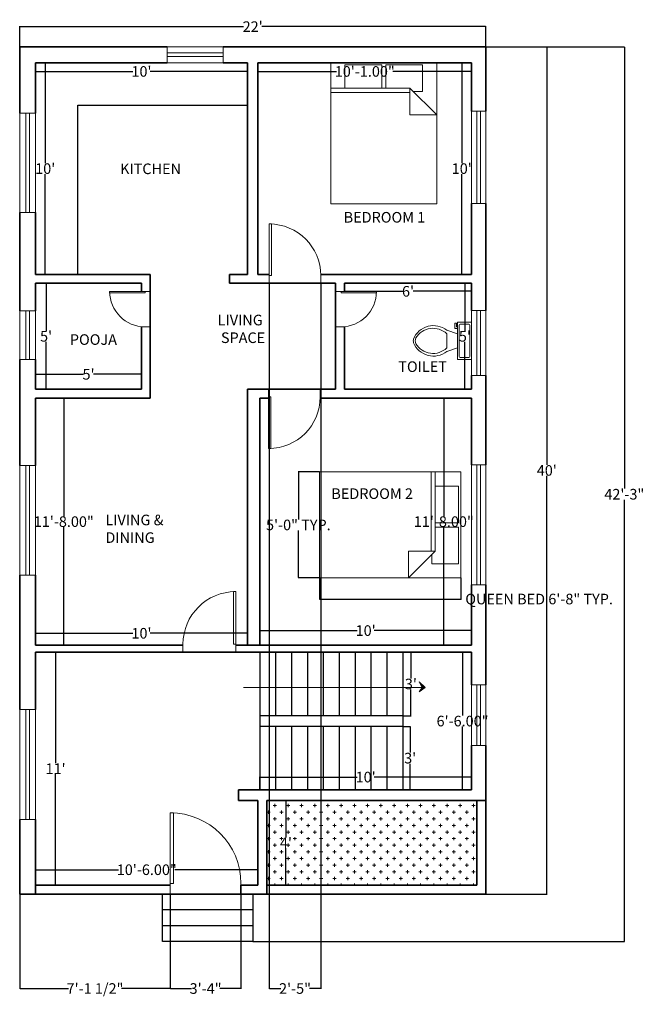
# Model space of a CAD drawing. Units: inches. Extents: x 14 to 1508, y -30 to 806.
# Tile 4 of 4: x 1154 to 1508, y -30 to 528. Entities that reach past the tile are written whole.
import ezdxf

# ---------------------------------------------------------------- set-up
doc = ezdxf.new("R2010")
doc.units = ezdxf.units.IN
doc.header["$MEASUREMENT"] = 0
for name, color, linetype, lineweight in [('A-ANNO-DIMS', 6, 'Continuous', 18), ('A-ANNO-SYMB', 2, 'Continuous', 18), ('A-AREA-IDEN', 3, 'Continuous', 18), ('A-DOOR', 4, 'Continuous', 18), ('A-FLOR-CASE', 8, 'Continuous', 25), ('A-FLOR-FIXT', 8, 'Continuous', 18), ('A-FLOR-PATT', 3, 'Continuous', 13), ('A-FLOR-STRS', 7, 'Continuous', 25), ('A-FURN', 8, 'Continuous', 18), ('A-GLAZ', 4, 'Continuous', 18), ('A-WALL', 7, 'Continuous', 35)]:
    doc.layers.add(name, color=color, linetype=linetype, lineweight=lineweight)
doc.styles.get("Standard").update_dxf_attribs({"font": 'arial.ttf'})
doc.dimstyles.get("Standard").update_dxf_attribs({"dimtxt": 6, "dimasz": 0.18, "dimexe": 0.18, "dimexo": 0.0625, "dimgap": 0.09, "dimtad": 0, "dimtih": 1, "dimtoh": 1, "dimzin": 0, "dimdsep": 46, "dimlunit": 3, "dimtxsty": 'Standard', "dimcen": 0.09, "dimadec": 0, "dimazin": 0, "dimtfac": 1, "dimtofl": 0, "dimtmove": 0, "dimatfit": 3, "dimfxl": 1, "dimtolj": 1, "dimtzin": 0, "dimarcsym": 0})

# ---------------------------------------------------------------- blocks, each defined once
blk = doc.blocks.new('*D55')
at = {"layer": 'A-ANNO-DIMS', "color": 0, "lineweight": -2, "transparency": 16777216}
for p, q in [((1370.88, 169.37), (1375.62, 169.37)), ((1375.44, 169.19), (1375.44, 154.52)), ((1375.44, 133.55), (1375.44, 148.21)), ((1370.88, 133.37), (1375.62, 133.37))]:
    blk.add_line(p, q, dxfattribs=at)
at = {"layer": 'A-ANNO-DIMS', "color": 0, "transparency": 16777216}
for points in [[(1375.41, 169.19), (1375.47, 169.19), (1375.44, 169.37)], [(1375.41, 133.55), (1375.47, 133.55), (1375.44, 133.37)]]:
    blk.add_solid(points, dxfattribs=at)
at = {"layer": 'Defpoints', "color": 0, "transparency": 16777216}
for p in [(1370.82, 169.37), (1375.44, 169.37), (1370.82, 133.37)]:
    blk.add_point(p, dxfattribs=at)
at = {"layer": 'A-ANNO-DIMS', "color": 0, "transparency": 16777216, "insert": (1375.44, 151.37), "char_height": 6, "attachment_point": 5}
blk.add_mtext("\\A1;3'", dxfattribs=at)
blk = doc.blocks.new('*D56')
at = {"layer": 'A-ANNO-DIMS', "color": 0, "lineweight": -2, "transparency": 16777216}
for p, q in [((1370.88, 127.37), (1375.22, 127.37)), ((1375.04, 127.19), (1375.04, 112.52)), ((1375.04, 91.55), (1375.04, 106.21)), ((1370.88, 91.37), (1375.22, 91.37))]:
    blk.add_line(p, q, dxfattribs=at)
at = {"layer": 'A-ANNO-DIMS', "color": 0, "transparency": 16777216}
for points in [[(1375.01, 127.19), (1375.07, 127.19), (1375.04, 127.37)], [(1375.01, 91.55), (1375.07, 91.55), (1375.04, 91.37)]]:
    blk.add_solid(points, dxfattribs=at)
at = {"layer": 'Defpoints', "color": 0, "transparency": 16777216}
for p in [(1370.82, 127.37), (1370.82, 91.37), (1375.04, 91.37)]:
    blk.add_point(p, dxfattribs=at)
at = {"layer": 'A-ANNO-DIMS', "color": 0, "transparency": 16777216, "insert": (1375.04, 109.37), "char_height": 6, "attachment_point": 5}
blk.add_mtext("\\A1;3'", dxfattribs=at)
blk = doc.blocks.new('*D57')
at = {"layer": 'A-ANNO-DIMS', "color": 0, "lineweight": -2, "transparency": 16777216}
for p, q in [((1409.76, 169.37), (1404.53, 169.37)), ((1404.71, 169.19), (1404.71, 133.52)), ((1404.71, 91.55), (1404.71, 127.22)), ((1409.76, 91.37), (1404.53, 91.37))]:
    blk.add_line(p, q, dxfattribs=at)
at = {"layer": 'A-ANNO-DIMS', "color": 0, "transparency": 16777216}
for points in [[(1404.68, 169.19), (1404.74, 169.19), (1404.71, 169.37)], [(1404.68, 91.55), (1404.74, 91.55), (1404.71, 91.37)]]:
    blk.add_solid(points, dxfattribs=at)
at = {"layer": 'Defpoints', "color": 0, "transparency": 16777216}
for p in [(1404.71, 169.37), (1409.82, 169.37), (1409.82, 91.37)]:
    blk.add_point(p, dxfattribs=at)
at = {"layer": 'A-ANNO-DIMS', "color": 0, "transparency": 16777216, "insert": (1404.71, 130.37), "char_height": 6, "attachment_point": 5}
blk.add_mtext('\\A1;6\'-6.00"', dxfattribs=at)
blk = doc.blocks.new('*D58')
at = {"layer": 'A-ANNO-DIMS', "color": 0, "lineweight": -2, "transparency": 16777216}
for p, q in [((1289.82, 91.43), (1289.82, 98.81)), ((1290, 98.63), (1344.92, 98.63)), ((1409.64, 98.63), (1354.72, 98.63)), ((1409.82, 91.43), (1409.82, 98.81))]:
    blk.add_line(p, q, dxfattribs=at)
at = {"layer": 'A-ANNO-DIMS', "color": 0, "transparency": 16777216}
for points in [[(1290, 98.66), (1290, 98.6), (1289.82, 98.63)], [(1409.64, 98.66), (1409.64, 98.6), (1409.82, 98.63)]]:
    blk.add_solid(points, dxfattribs=at)
at = {"layer": 'Defpoints', "color": 0, "transparency": 16777216}
for p in [(1289.82, 98.63), (1289.82, 91.37), (1409.82, 91.37)]:
    blk.add_point(p, dxfattribs=at)
at = {"layer": 'A-ANNO-DIMS', "color": 0, "transparency": 16777216, "insert": (1349.82, 98.63), "char_height": 6, "attachment_point": 5}
blk.add_mtext("\\A1;10'", dxfattribs=at)
blk = doc.blocks.new('*U61')
for p, q in [((0, 0), (0, -6)), ((40, 0), (40, -6))]:
    blk.add_line(p, q)
blk.add_lwpolyline([(0, 0), (0, 40), (1.75, 40), (1.75, 0)], close=True)
blk.add_arc((0, 0), 40, 0, 90)
blk = doc.blocks.new('Bed - Queen')
for p, q in [((0, -80.00003), (0, 0)), ((0, 0), (59.99999, 0)), ((59.99999, 0), (59.99999, -80.00003)), ((7.99999, -1.2), (28.79998, -1.2)), ((7.99999, -14.4), (7.99999, -1.2)), ((28.79998, -1.2), (28.79998, -14.4)), ((31.19999, -1.2), (51.99999, -1.2)), ((31.19999, -14.4), (31.19999, -1.2)), ((51.99999, -1.2), (51.99999, -16.4)), ((0, -14.4), (44.8, -14.4)), ((59.99999, -29.6), (44.8, -14.4)), ((44.8, -14.4), (44.8, -29.6)), ((51.99999, -16.4), (46.79936, -16.4)), ((44.8, -16.8), (0, -16.8)), ((44.8, -29.6), (59.99999, -29.6)), ((59.99999, -80.00003), (0, -80.00003))]:
    blk.add_line(p, q)
blk = doc.blocks.new('*U63')
for p, q in [((9.5, -6), (9.5, -2)), ((-10, -8.5), (-8, -8.5)), ((-10, -9.5), (-10, -8.5)), ((-7, -9.5), (-10, -9.5)), ((-8, -8.5), (-8, -8)), ((-7, -8), (-7, -9.5)), ((-4, -8), (-6, -14)), ((4, -8), (6, -14)), ((4, -14), (-4, -14))]:
    blk.add_line(p, q)
blk.add_lwpolyline([(10.5, -8), (10.5, 0), (-10.5, 0), (-10.5, -8)], close=True)
for points in [[(-9.5, -2), (-9.5, -6)], [(8.5, -1), (-8.5, -1)], [(-8.5, -7), (8.5, -7)]]:
    blk.add_lwpolyline(points)
for centre, radius, start, end in [((-8.62, -1.88), 0.884, 81.8699, 188.1301), ((8.62, -1.88), 0.884, 351.8699, 98.1301), ((-8.62, -6.12), 0.884, 171.8699, 278.1301), ((8.62, -6.12), 0.884, 261.8699, 8.1301), ((3.52, -21.58), 12.17, 141.4691, 247.9714), ((4.2, -21.82), 11.33, 136.3677, 238.9468), ((-3.52, -21.58), 12.17, 292.0284, 38.5307), ((-4.2, -21.82), 11.33, 301.053, 43.6321), ((0, -27.88), 4, 245.7318, 294.2682), ((0, -29), 4, 254.8605, 285.1395)]:
    blk.add_arc(centre, radius, start, end)
blk = doc.blocks.new('*D64')
at = {"layer": 'A-ANNO-DIMS', "color": 0, "lineweight": -2, "transparency": 16777216}
for p, q in [((1293.88, 85.37), (1304.84, 85.37)), ((1304.66, 85.19), (1304.66, 64.46)), ((1304.66, 37.55), (1304.66, 58.28)), ((1293.88, 37.37), (1304.84, 37.37))]:
    blk.add_line(p, q, dxfattribs=at)
at = {"layer": 'A-ANNO-DIMS', "color": 0, "transparency": 16777216}
for points in [[(1304.63, 85.19), (1304.69, 85.19), (1304.66, 85.37)], [(1304.63, 37.55), (1304.69, 37.55), (1304.66, 37.37)]]:
    blk.add_solid(points, dxfattribs=at)
at = {"layer": 'Defpoints', "color": 0, "transparency": 16777216}
for p in [(1293.82, 85.37), (1293.82, 37.37), (1304.66, 37.37)]:
    blk.add_point(p, dxfattribs=at)
at = {"layer": 'A-ANNO-DIMS', "color": 0, "transparency": 16777216, "insert": (1304.66, 61.37), "char_height": 6, "attachment_point": 5}
blk.add_mtext("\\A1;4'", dxfattribs=at)
blk = doc.blocks.new('*D65')
at = {"layer": 'A-ANNO-DIMS', "color": 0, "lineweight": -2, "transparency": 16777216}
for p, q in [((1162.88, 169.37), (1174.32, 169.37)), ((1174.14, 169.19), (1174.14, 106.47)), ((1174.14, 37.55), (1174.14, 100.27)), ((1162.88, 37.37), (1174.32, 37.37))]:
    blk.add_line(p, q, dxfattribs=at)
at = {"layer": 'A-ANNO-DIMS', "color": 0, "transparency": 16777216}
for points in [[(1174.11, 169.19), (1174.17, 169.19), (1174.14, 169.37)], [(1174.11, 37.55), (1174.17, 37.55), (1174.14, 37.37)]]:
    blk.add_solid(points, dxfattribs=at)
at = {"layer": 'Defpoints', "color": 0, "transparency": 16777216}
for p in [(1162.82, 169.37), (1162.82, 37.37), (1174.14, 37.37)]:
    blk.add_point(p, dxfattribs=at)
at = {"layer": 'A-ANNO-DIMS', "color": 0, "transparency": 16777216, "insert": (1174.14, 103.37), "char_height": 6, "attachment_point": 5}
blk.add_mtext("\\A1;11'", dxfattribs=at)
blk = doc.blocks.new('*D66')
at = {"layer": 'A-ANNO-DIMS', "color": 0, "lineweight": -2, "transparency": 16777216}
for p, q in [((1162.82, 37.43), (1162.82, 46.33)), ((1163, 46.15), (1209.88, 46.15)), ((1288.64, 46.15), (1241.76, 46.15)), ((1288.82, 37.43), (1288.82, 46.33))]:
    blk.add_line(p, q, dxfattribs=at)
at = {"layer": 'A-ANNO-DIMS', "color": 0, "transparency": 16777216}
for points in [[(1163, 46.18), (1163, 46.12), (1162.82, 46.15)], [(1288.64, 46.18), (1288.64, 46.12), (1288.82, 46.15)]]:
    blk.add_solid(points, dxfattribs=at)
at = {"layer": 'Defpoints', "color": 0, "transparency": 16777216}
for p in [(1288.82, 46.15), (1162.82, 37.37), (1288.82, 37.37)]:
    blk.add_point(p, dxfattribs=at)
at = {"layer": 'A-ANNO-DIMS', "color": 0, "transparency": 16777216, "insert": (1225.82, 46.15), "char_height": 6, "attachment_point": 5}
blk.add_mtext('\\A1;10\'-6.00"', dxfattribs=at)
blk = doc.blocks.new('*D67')
at = {"layer": 'A-ANNO-DIMS', "color": 0, "lineweight": -2, "transparency": 16777216}
for p, q in [((1162.82, 173.43), (1162.82, 180.28)), ((1163, 180.1), (1217.92, 180.1)), ((1282.64, 180.1), (1227.72, 180.1)), ((1282.82, 173.43), (1282.82, 180.28))]:
    blk.add_line(p, q, dxfattribs=at)
at = {"layer": 'A-ANNO-DIMS', "color": 0, "transparency": 16777216}
for points in [[(1163, 180.13), (1163, 180.07), (1162.82, 180.1)], [(1282.64, 180.13), (1282.64, 180.07), (1282.82, 180.1)]]:
    blk.add_solid(points, dxfattribs=at)
at = {"layer": 'Defpoints', "color": 0, "transparency": 16777216}
for p in [(1282.82, 180.1), (1162.82, 173.37), (1282.82, 173.37)]:
    blk.add_point(p, dxfattribs=at)
at = {"layer": 'A-ANNO-DIMS', "color": 0, "transparency": 16777216, "insert": (1222.82, 180.1), "char_height": 6, "attachment_point": 5}
blk.add_mtext("\\A1;10'", dxfattribs=at)
blk = doc.blocks.new('*D68')
at = {"layer": 'A-ANNO-DIMS', "color": 0, "lineweight": -2, "transparency": 16777216}
for p, q in [((1162.88, 313.37), (1178.98, 313.37)), ((1178.8, 313.19), (1178.8, 246.52)), ((1178.8, 173.55), (1178.8, 240.22)), ((1162.88, 173.37), (1178.98, 173.37))]:
    blk.add_line(p, q, dxfattribs=at)
at = {"layer": 'A-ANNO-DIMS', "color": 0, "transparency": 16777216}
for points in [[(1178.77, 313.19), (1178.83, 313.19), (1178.8, 313.37)], [(1178.77, 173.55), (1178.83, 173.55), (1178.8, 173.37)]]:
    blk.add_solid(points, dxfattribs=at)
at = {"layer": 'Defpoints', "color": 0, "transparency": 16777216}
for p in [(1162.82, 313.37), (1162.82, 173.37), (1178.8, 173.37)]:
    blk.add_point(p, dxfattribs=at)
at = {"layer": 'A-ANNO-DIMS', "color": 0, "transparency": 16777216, "insert": (1178.8, 243.37), "char_height": 6, "attachment_point": 5}
blk.add_mtext('\\A1;11\'-8.00"', dxfattribs=at)
blk = doc.blocks.new('*D69')
at = {"layer": 'A-ANNO-DIMS', "color": 0, "lineweight": -2, "transparency": 16777216}
for p, q in [((1289.82, 173.43), (1289.82, 181.82)), ((1290, 181.64), (1344.92, 181.64)), ((1409.64, 181.64), (1354.72, 181.64)), ((1409.82, 173.43), (1409.82, 181.82))]:
    blk.add_line(p, q, dxfattribs=at)
at = {"layer": 'A-ANNO-DIMS', "color": 0, "transparency": 16777216}
for points in [[(1290, 181.67), (1290, 181.61), (1289.82, 181.64)], [(1409.64, 181.67), (1409.64, 181.61), (1409.82, 181.64)]]:
    blk.add_solid(points, dxfattribs=at)
at = {"layer": 'Defpoints', "color": 0, "transparency": 16777216}
for p in [(1409.82, 181.64), (1289.82, 173.37), (1409.82, 173.37)]:
    blk.add_point(p, dxfattribs=at)
at = {"layer": 'A-ANNO-DIMS', "color": 0, "transparency": 16777216, "insert": (1349.82, 181.64), "char_height": 6, "attachment_point": 5}
blk.add_mtext("\\A1;10'", dxfattribs=at)
blk = doc.blocks.new('*D70')
at = {"layer": 'A-ANNO-DIMS', "color": 0, "lineweight": -2, "transparency": 16777216}
for p, q in [((1409.76, 313.37), (1393.91, 313.37)), ((1394.09, 313.19), (1394.09, 246.52)), ((1394.09, 173.55), (1394.09, 240.22)), ((1409.76, 173.37), (1393.91, 173.37))]:
    blk.add_line(p, q, dxfattribs=at)
at = {"layer": 'A-ANNO-DIMS', "color": 0, "transparency": 16777216}
for points in [[(1394.06, 313.19), (1394.12, 313.19), (1394.09, 313.37)], [(1394.06, 173.55), (1394.12, 173.55), (1394.09, 173.37)]]:
    blk.add_solid(points, dxfattribs=at)
at = {"layer": 'Defpoints', "color": 0, "transparency": 16777216}
for p in [(1394.09, 313.37), (1409.82, 313.37), (1409.82, 173.37)]:
    blk.add_point(p, dxfattribs=at)
at = {"layer": 'A-ANNO-DIMS', "color": 0, "transparency": 16777216, "insert": (1394.09, 243.37), "char_height": 6, "attachment_point": 5}
blk.add_mtext('\\A1;11\'-8.00"', dxfattribs=at)
blk = doc.blocks.new('*D71')
at = {"layer": 'A-ANNO-DIMS', "color": 0, "lineweight": -2, "transparency": 16777216}
for p, q in [((1162.82, 318.43), (1162.82, 327.02)), ((1163, 326.84), (1189.97, 326.84)), ((1222.64, 326.84), (1195.67, 326.84)), ((1222.82, 318.43), (1222.82, 327.02))]:
    blk.add_line(p, q, dxfattribs=at)
at = {"layer": 'A-ANNO-DIMS', "color": 0, "transparency": 16777216}
for points in [[(1163, 326.87), (1163, 326.81), (1162.82, 326.84)], [(1222.64, 326.87), (1222.64, 326.81), (1222.82, 326.84)]]:
    blk.add_solid(points, dxfattribs=at)
at = {"layer": 'Defpoints', "color": 0, "transparency": 16777216}
for p in [(1222.82, 326.84), (1162.82, 318.37), (1222.82, 318.37)]:
    blk.add_point(p, dxfattribs=at)
at = {"layer": 'A-ANNO-DIMS', "color": 0, "transparency": 16777216, "insert": (1192.82, 326.84), "char_height": 6, "attachment_point": 5}
blk.add_mtext("\\A1;5'", dxfattribs=at)
blk = doc.blocks.new('*D72')
at = {"layer": 'A-ANNO-DIMS', "color": 0, "lineweight": -2, "transparency": 16777216}
for p, q in [((1162.88, 378.37), (1168.95, 378.37)), ((1168.77, 378.19), (1168.77, 351.51)), ((1168.77, 318.55), (1168.77, 345.23)), ((1162.88, 318.37), (1168.95, 318.37))]:
    blk.add_line(p, q, dxfattribs=at)
at = {"layer": 'A-ANNO-DIMS', "color": 0, "transparency": 16777216}
for points in [[(1168.74, 378.19), (1168.8, 378.19), (1168.77, 378.37)], [(1168.74, 318.55), (1168.8, 318.55), (1168.77, 318.37)]]:
    blk.add_solid(points, dxfattribs=at)
at = {"layer": 'Defpoints', "color": 0, "transparency": 16777216}
for p in [(1162.82, 378.37), (1162.82, 318.37), (1168.77, 318.37)]:
    blk.add_point(p, dxfattribs=at)
at = {"layer": 'A-ANNO-DIMS', "color": 0, "transparency": 16777216, "insert": (1168.77, 348.37), "char_height": 6, "attachment_point": 5}
blk.add_mtext("\\A1;5'", dxfattribs=at)
blk = doc.blocks.new('*D73')
at = {"layer": 'A-ANNO-DIMS', "color": 0, "lineweight": -2, "transparency": 16777216}
for p, q in [((1337.82, 378.31), (1337.82, 373.67)), ((1338, 373.85), (1370.95, 373.85)), ((1409.64, 373.85), (1376.69, 373.85)), ((1409.82, 378.31), (1409.82, 373.67))]:
    blk.add_line(p, q, dxfattribs=at)
at = {"layer": 'A-ANNO-DIMS', "color": 0, "transparency": 16777216}
for points in [[(1338, 373.88), (1338, 373.82), (1337.82, 373.85)], [(1409.64, 373.88), (1409.64, 373.82), (1409.82, 373.85)]]:
    blk.add_solid(points, dxfattribs=at)
at = {"layer": 'Defpoints', "color": 0, "transparency": 16777216}
for p in [(1337.82, 378.37), (1409.82, 378.37), (1409.82, 373.85)]:
    blk.add_point(p, dxfattribs=at)
at = {"layer": 'A-ANNO-DIMS', "color": 0, "transparency": 16777216, "insert": (1373.82, 373.85), "char_height": 6, "attachment_point": 5}
blk.add_mtext("\\A1;6'", dxfattribs=at)
blk = doc.blocks.new('*D74')
at = {"layer": 'A-ANNO-DIMS', "color": 0, "lineweight": -2, "transparency": 16777216}
for p, q in [((1409.76, 378.37), (1405.85, 378.37)), ((1406.03, 378.19), (1406.03, 351.51)), ((1406.03, 318.55), (1406.03, 345.23)), ((1409.76, 318.37), (1405.85, 318.37))]:
    blk.add_line(p, q, dxfattribs=at)
at = {"layer": 'A-ANNO-DIMS', "color": 0, "transparency": 16777216}
for points in [[(1406, 378.19), (1406.06, 378.19), (1406.03, 378.37)], [(1406, 318.55), (1406.06, 318.55), (1406.03, 318.37)]]:
    blk.add_solid(points, dxfattribs=at)
at = {"layer": 'Defpoints', "color": 0, "transparency": 16777216}
for p in [(1406.03, 378.37), (1409.82, 378.37), (1409.82, 318.37)]:
    blk.add_point(p, dxfattribs=at)
at = {"layer": 'A-ANNO-DIMS', "color": 0, "transparency": 16777216, "insert": (1406.03, 348.37), "char_height": 6, "attachment_point": 5}
blk.add_mtext("\\A1;5'", dxfattribs=at)
blk = doc.blocks.new('*D75')
at = {"layer": 'A-ANNO-DIMS', "color": 0, "lineweight": -2, "transparency": 16777216}
for p, q in [((1162.82, 503.31), (1162.82, 498.24)), ((1282.82, 503.31), (1282.82, 498.24)), ((1163, 498.42), (1217.92, 498.42)), ((1282.64, 498.42), (1227.72, 498.42))]:
    blk.add_line(p, q, dxfattribs=at)
at = {"layer": 'A-ANNO-DIMS', "color": 0, "transparency": 16777216}
for points in [[(1163, 498.45), (1163, 498.39), (1162.82, 498.42)], [(1282.64, 498.45), (1282.64, 498.39), (1282.82, 498.42)]]:
    blk.add_solid(points, dxfattribs=at)
at = {"layer": 'Defpoints', "color": 0, "transparency": 16777216}
for p in [(1162.82, 503.37), (1282.82, 503.37), (1282.82, 498.42)]:
    blk.add_point(p, dxfattribs=at)
at = {"layer": 'A-ANNO-DIMS', "color": 0, "transparency": 16777216, "insert": (1222.82, 498.42), "char_height": 6, "attachment_point": 5}
blk.add_mtext("\\A1;10'", dxfattribs=at)
blk = doc.blocks.new('*D76')
at = {"layer": 'A-ANNO-DIMS', "color": 0, "lineweight": -2, "transparency": 16777216}
for p, q in [((1162.88, 503.37), (1168.47, 503.37)), ((1168.29, 503.19), (1168.29, 446.52)), ((1168.29, 383.55), (1168.29, 440.22)), ((1162.88, 383.37), (1168.47, 383.37))]:
    blk.add_line(p, q, dxfattribs=at)
at = {"layer": 'A-ANNO-DIMS', "color": 0, "transparency": 16777216}
for points in [[(1168.26, 503.19), (1168.32, 503.19), (1168.29, 503.37)], [(1168.26, 383.55), (1168.32, 383.55), (1168.29, 383.37)]]:
    blk.add_solid(points, dxfattribs=at)
at = {"layer": 'Defpoints', "color": 0, "transparency": 16777216}
for p in [(1162.82, 503.37), (1168.29, 503.37), (1162.82, 383.37)]:
    blk.add_point(p, dxfattribs=at)
at = {"layer": 'A-ANNO-DIMS', "color": 0, "transparency": 16777216, "insert": (1168.29, 443.37), "char_height": 6, "attachment_point": 5}
blk.add_mtext("\\A1;10'", dxfattribs=at)
blk = doc.blocks.new('*D77')
at = {"layer": 'A-ANNO-DIMS', "color": 0, "lineweight": -2, "transparency": 16777216}
for p, q in [((1288.82, 503.31), (1288.82, 498.24)), ((1409.82, 503.31), (1409.82, 498.24)), ((1289, 498.42), (1333.38, 498.42)), ((1409.64, 498.42), (1365.26, 498.42))]:
    blk.add_line(p, q, dxfattribs=at)
at = {"layer": 'A-ANNO-DIMS', "color": 0, "transparency": 16777216}
for points in [[(1289, 498.45), (1289, 498.39), (1288.82, 498.42)], [(1409.64, 498.45), (1409.64, 498.39), (1409.82, 498.42)]]:
    blk.add_solid(points, dxfattribs=at)
at = {"layer": 'Defpoints', "color": 0, "transparency": 16777216}
for p in [(1288.82, 503.37), (1409.82, 503.37), (1409.82, 498.42)]:
    blk.add_point(p, dxfattribs=at)
at = {"layer": 'A-ANNO-DIMS', "color": 0, "transparency": 16777216, "insert": (1349.32, 498.42), "char_height": 6, "attachment_point": 5}
blk.add_mtext('\\A1;10\'-1.00"', dxfattribs=at)
blk = doc.blocks.new('*D78')
at = {"layer": 'A-ANNO-DIMS', "color": 0, "lineweight": -2, "transparency": 16777216}
for p, q in [((1409.76, 503.37), (1404.08, 503.37)), ((1404.26, 503.19), (1404.26, 446.52)), ((1404.26, 383.55), (1404.26, 440.22)), ((1409.76, 383.37), (1404.08, 383.37))]:
    blk.add_line(p, q, dxfattribs=at)
at = {"layer": 'A-ANNO-DIMS', "color": 0, "transparency": 16777216}
for points in [[(1404.23, 503.19), (1404.29, 503.19), (1404.26, 503.37)], [(1404.23, 383.55), (1404.29, 383.55), (1404.26, 383.37)]]:
    blk.add_solid(points, dxfattribs=at)
at = {"layer": 'Defpoints', "color": 0, "transparency": 16777216}
for p in [(1404.26, 503.37), (1409.82, 503.37), (1409.82, 383.37)]:
    blk.add_point(p, dxfattribs=at)
at = {"layer": 'A-ANNO-DIMS', "color": 0, "transparency": 16777216, "insert": (1404.26, 443.37), "char_height": 6, "attachment_point": 5}
blk.add_mtext("\\A1;10'", dxfattribs=at)
blk = doc.blocks.new('*D79')
at = {"layer": 'A-ANNO-DIMS', "color": 0, "lineweight": -2, "transparency": 16777216}
for p, q in [((1153.82, 512.43), (1153.82, 523.98)), ((1154, 523.8), (1280.59, 523.8)), ((1417.64, 523.8), (1291.05, 523.8)), ((1417.82, 512.43), (1417.82, 523.98))]:
    blk.add_line(p, q, dxfattribs=at)
at = {"layer": 'A-ANNO-DIMS', "color": 0, "transparency": 16777216}
for points in [[(1154, 523.83), (1154, 523.77), (1153.82, 523.8)], [(1417.64, 523.83), (1417.64, 523.77), (1417.82, 523.8)]]:
    blk.add_solid(points, dxfattribs=at)
at = {"layer": 'Defpoints', "color": 0, "transparency": 16777216}
for p in [(1417.82, 523.8), (1153.82, 512.37), (1417.82, 512.37)]:
    blk.add_point(p, dxfattribs=at)
at = {"layer": 'A-ANNO-DIMS', "color": 0, "transparency": 16777216, "insert": (1285.82, 523.8), "char_height": 6, "attachment_point": 5}
blk.add_mtext("\\A1;22'", dxfattribs=at)
blk = doc.blocks.new('*D80')
at = {"layer": 'A-ANNO-DIMS', "color": 0, "lineweight": -2, "transparency": 16777216}
for p, q in [((1417.88, 512.37), (1452.63, 512.37)), ((1452.45, 512.19), (1452.45, 275.52)), ((1452.45, 32.55), (1452.45, 269.22)), ((1417.88, 32.37), (1452.63, 32.37))]:
    blk.add_line(p, q, dxfattribs=at)
at = {"layer": 'A-ANNO-DIMS', "color": 0, "transparency": 16777216}
for points in [[(1452.42, 512.19), (1452.48, 512.19), (1452.45, 512.37)], [(1452.42, 32.55), (1452.48, 32.55), (1452.45, 32.37)]]:
    blk.add_solid(points, dxfattribs=at)
at = {"layer": 'Defpoints', "color": 0, "transparency": 16777216}
for p in [(1417.82, 512.37), (1417.82, 32.37), (1452.45, 32.37)]:
    blk.add_point(p, dxfattribs=at)
at = {"layer": 'A-ANNO-DIMS', "color": 0, "transparency": 16777216, "insert": (1452.45, 272.37), "char_height": 6, "attachment_point": 5}
blk.add_mtext("\\A1;40'", dxfattribs=at)
blk = doc.blocks.new('*D91')
at = {"layer": 'A-ANNO-DIMS', "color": 0, "lineweight": -2, "transparency": 16777216}
for p, q in [((1323.69, 211.43), (1323.69, 199.32)), ((1403.69, 211.43), (1403.69, 199.32)), ((1323.87, 199.5), (1403.51, 199.5)), ((1403.69, 199.5), (1403.87, 199.5))]:
    blk.add_line(p, q, dxfattribs=at)
at = {"layer": 'A-ANNO-DIMS', "color": 0, "transparency": 16777216}
for points in [[(1323.87, 199.53), (1323.87, 199.47), (1323.69, 199.5)], [(1403.51, 199.53), (1403.51, 199.47), (1403.69, 199.5)]]:
    blk.add_solid(points, dxfattribs=at)
at = {"layer": 'Defpoints', "color": 0, "transparency": 16777216}
for p in [(1323.69, 211.5), (1403.69, 211.5), (1403.69, 199.5)]:
    blk.add_point(p, dxfattribs=at)
at = {"layer": 'A-ANNO-DIMS', "color": 0, "transparency": 16777216, "insert": (1448.09, 199.5), "char_height": 6, "attachment_point": 5}
blk.add_mtext('\\A1;QUEEN BED 6\'-8" TYP.', dxfattribs=at)
blk = doc.blocks.new('*D92')
at = {"layer": 'A-ANNO-DIMS', "color": 0, "lineweight": -2, "transparency": 16777216}
for p, q in [((1323.63, 271.5), (1311.51, 271.5)), ((1311.69, 271.32), (1311.69, 244.65)), ((1311.69, 211.68), (1311.69, 238.34)), ((1323.63, 211.5), (1311.51, 211.5))]:
    blk.add_line(p, q, dxfattribs=at)
at = {"layer": 'A-ANNO-DIMS', "color": 0, "transparency": 16777216}
for points in [[(1311.66, 271.32), (1311.72, 271.32), (1311.69, 271.5)], [(1311.66, 211.68), (1311.72, 211.68), (1311.69, 211.5)]]:
    blk.add_solid(points, dxfattribs=at)
at = {"layer": 'Defpoints', "color": 0, "transparency": 16777216}
for p in [(1323.69, 271.5), (1311.69, 211.5), (1323.69, 211.5)]:
    blk.add_point(p, dxfattribs=at)
at = {"layer": 'A-ANNO-DIMS', "color": 0, "transparency": 16777216, "insert": (1311.69, 241.5), "char_height": 6, "attachment_point": 5}
blk.add_mtext('\\A1;5\'-0" TYP.', dxfattribs=at)
blk = doc.blocks.new('*D109')
at = {"layer": 'A-ANNO-DIMS', "color": 0, "lineweight": -2, "transparency": 16777216}
for p, q in [((1417.88, 512.37), (1496.55, 512.37)), ((1496.37, 512.19), (1496.37, 262.04)), ((1496.37, 5.58), (1496.37, 255.73)), ((1285.88, 5.4), (1496.55, 5.4))]:
    blk.add_line(p, q, dxfattribs=at)
at = {"layer": 'A-ANNO-DIMS', "color": 0, "transparency": 16777216}
for points in [[(1496.34, 512.19), (1496.4, 512.19), (1496.37, 512.37)], [(1496.34, 5.58), (1496.4, 5.58), (1496.37, 5.4)]]:
    blk.add_solid(points, dxfattribs=at)
at = {"layer": 'Defpoints', "color": 0, "transparency": 16777216}
for p in [(1417.82, 512.37), (1496.37, 512.37), (1285.82, 5.4)]:
    blk.add_point(p, dxfattribs=at)
at = {"layer": 'A-ANNO-DIMS', "color": 0, "transparency": 16777216, "insert": (1496.37, 258.89), "char_height": 6, "attachment_point": 5}
blk.add_mtext('\\A1;42\'-3"', dxfattribs=at)
blk = doc.blocks.new('*D110')
at = {"layer": 'A-ANNO-DIMS', "color": 0, "lineweight": -2, "transparency": 16777216}
for p, q in [((1239.13, 32.31), (1239.13, -21.33)), ((1279.15, 32.31), (1279.15, -21.33)), ((1239.31, -21.15), (1251.08, -21.15)), ((1278.97, -21.15), (1267.2, -21.15))]:
    blk.add_line(p, q, dxfattribs=at)
at = {"layer": 'A-ANNO-DIMS', "color": 0, "transparency": 16777216}
for points in [[(1239.31, -21.12), (1239.31, -21.18), (1239.13, -21.15)], [(1278.97, -21.12), (1278.97, -21.18), (1279.15, -21.15)]]:
    blk.add_solid(points, dxfattribs=at)
at = {"layer": 'Defpoints', "color": 0, "transparency": 16777216}
for p in [(1239.13, 32.37), (1279.15, 32.37), (1279.15, -21.15)]:
    blk.add_point(p, dxfattribs=at)
at = {"layer": 'A-ANNO-DIMS', "color": 0, "transparency": 16777216, "insert": (1259.14, -21.15), "char_height": 6, "attachment_point": 5}
blk.add_mtext('\\A1;3\'-4"', dxfattribs=at)
blk = doc.blocks.new('*D111')
at = {"layer": 'A-ANNO-DIMS', "color": 0, "lineweight": -2, "transparency": 16777216}
for p, q in [((1153.82, 32.31), (1153.82, -21.33)), ((1239.13, 32.31), (1239.13, -21.33)), ((1154, -21.15), (1181.45, -21.15)), ((1238.95, -21.15), (1211.51, -21.15))]:
    blk.add_line(p, q, dxfattribs=at)
at = {"layer": 'A-ANNO-DIMS', "color": 0, "transparency": 16777216}
for points in [[(1154, -21.12), (1154, -21.18), (1153.82, -21.15)], [(1238.95, -21.12), (1238.95, -21.18), (1239.13, -21.15)]]:
    blk.add_solid(points, dxfattribs=at)
at = {"layer": 'Defpoints', "color": 0, "transparency": 16777216}
for p in [(1153.82, 32.37), (1239.13, 32.37), (1239.13, -21.15)]:
    blk.add_point(p, dxfattribs=at)
at = {"layer": 'A-ANNO-DIMS', "color": 0, "transparency": 16777216, "insert": (1196.48, -21.15), "char_height": 6, "attachment_point": 5}
blk.add_mtext('\\A1;7\'-1 1/2"', dxfattribs=at)
blk = doc.blocks.new('*D112')
at = {"layer": 'A-ANNO-DIMS', "color": 0, "lineweight": -2, "transparency": 16777216}
for p, q in [((1295.21, 378.37), (1295.21, -21.33)), ((1324.41, 378.37), (1324.41, -21.33)), ((1295.39, -21.15), (1301.69, -21.15)), ((1324.23, -21.15), (1317.92, -21.15))]:
    blk.add_line(p, q, dxfattribs=at)
at = {"layer": 'A-ANNO-DIMS', "color": 0, "transparency": 16777216}
for points in [[(1295.39, -21.12), (1295.39, -21.18), (1295.21, -21.15)], [(1324.23, -21.12), (1324.23, -21.18), (1324.41, -21.15)]]:
    blk.add_solid(points, dxfattribs=at)
at = {"layer": 'Defpoints', "color": 0, "transparency": 16777216}
for p in [(1295.21, 378.43), (1324.41, 378.43), (1324.41, -21.15)]:
    blk.add_point(p, dxfattribs=at)
at = {"layer": 'A-ANNO-DIMS', "color": 0, "transparency": 16777216, "insert": (1309.81, -21.15), "char_height": 6, "attachment_point": 5}
blk.add_mtext('\\A1;2\'-5"', dxfattribs=at)

msp = doc.modelspace()

# ---------------------------------------------------------------- hatches: boundary and pattern name
at = {"layer": 'A-ANNO-SYMB'}
h = msp.add_hatch(color=256, dxfattribs=at)
h.dxf.hatch_style = 1
h.paths.add_polyline_path([(1381.748, 149.483), (1380.121, 146.918), (1383.467, 149.483), (1380.067, 152.542)])
at = {"layer": 'A-FLOR-PATT'}
h = msp.add_hatch(dxfattribs=at)
h.set_pattern_fill('CROSS', color=256, scale=15)
h.paths.add_polyline_path([(1293.821, 85.369), (1293.821, 37.369), (1412.821, 37.369), (1412.821, 85.369)])

# ---------------------------------------------------------------- linework, layer by layer
at = {"layer": 'A-ANNO-SYMB'}
for p, q in [((1383.467, 149.483), (1380.067, 152.542)), ((1381.748, 149.483), (1380.067, 152.542)), ((1280.632, 149.483), (1381.748, 149.483)), ((1383.467, 149.483), (1380.121, 146.918)), ((1380.121, 146.918), (1381.748, 149.483))]:
    msp.add_line(p, q, dxfattribs=at)
at = {"layer": 'A-FLOR-CASE'}
for points in [[(1186.821, 474.831), (1186.821, 479.369)], [(1186.821, 479.369), (1282.821, 479.369)], [(1186.821, 383.369), (1186.821, 479.369)]]:
    msp.add_lwpolyline(points, dxfattribs=at)
at = {"layer": 'A-FLOR-STRS'}
for p, q in [((1234.779, 5.403), (1234.779, 32.369)), ((1285.821, 32.369), (1285.821, 5.403)), ((1285.821, 23.403), (1234.779, 23.403)), ((1285.821, 14.403), (1234.779, 14.403)), ((1285.821, 5.403), (1234.779, 5.403))]:
    msp.add_line(p, q, dxfattribs=at)
for points in [[(1289.821, 169.369), (1289.821, 91.369)], [(1298.821, 169.369), (1298.821, 133.369)], [(1307.821, 169.369), (1307.821, 133.369)], [(1316.821, 169.369), (1316.821, 133.369)], [(1325.821, 169.369), (1325.821, 133.369)], [(1334.821, 169.369), (1334.821, 133.369)], [(1343.821, 169.369), (1343.821, 133.369)], [(1352.821, 169.369), (1352.821, 133.369)], [(1361.821, 169.369), (1361.821, 133.369)], [(1370.821, 169.369), (1370.821, 91.369)], [(1370.821, 133.369), (1289.821, 133.369)], [(1370.821, 127.369), (1289.821, 127.369)], [(1298.821, 127.369), (1298.821, 91.369)], [(1307.821, 127.369), (1307.821, 91.369)], [(1316.821, 127.369), (1316.821, 91.369)], [(1325.821, 127.369), (1325.821, 91.369)], [(1334.821, 127.369), (1334.821, 91.369)], [(1343.821, 127.369), (1343.821, 91.369)], [(1352.821, 127.369), (1352.821, 91.369)], [(1361.821, 127.369), (1361.821, 91.369)]]:
    msp.add_lwpolyline(points, dxfattribs=at)
at = {"layer": 'A-GLAZ'}
for p, q in [((1237.371, 508.869), (1269.089, 508.869)), ((1237.371, 506.869), (1269.089, 506.869)), ((1157.321, 418.556), (1157.321, 474.831)), ((1159.321, 418.556), (1159.321, 474.831)), ((1412.821, 475.857), (1412.821, 423.507)), ((1414.821, 475.857), (1414.821, 423.507)), ((1157.321, 335.25), (1157.321, 362.705)), ((1159.321, 335.25), (1159.321, 362.705)), ((1412.821, 362.958), (1412.821, 326.158)), ((1414.821, 362.958), (1414.821, 326.158)), ((1157.321, 213.042), (1157.321, 275.143)), ((1159.321, 213.042), (1159.321, 275.143)), ((1412.821, 275.499), (1412.821, 207.634)), ((1414.821, 275.499), (1414.821, 207.634)), ((1412.821, 150.846), (1412.821, 116.447)), ((1414.821, 150.846), (1414.821, 116.447)), ((1157.321, 74.535), (1157.321, 136.837)), ((1159.321, 74.535), (1159.321, 136.837))]:
    msp.add_line(p, q, dxfattribs=at)
for points in [[(1237.371, 512.369), (1269.089, 512.369), (1269.089, 503.369), (1237.371, 503.369)], [(1153.821, 474.831), (1162.821, 474.831), (1162.821, 418.556), (1153.821, 418.556)], [(1409.821, 475.857), (1417.821, 475.857), (1417.821, 423.507), (1409.821, 423.507)], [(1153.821, 362.705), (1162.821, 362.705), (1162.821, 335.25), (1153.821, 335.25)], [(1409.821, 362.958), (1417.821, 362.958), (1417.821, 326.158), (1409.821, 326.158)], [(1153.821, 275.143), (1162.821, 275.143), (1162.821, 213.042), (1153.821, 213.042)], [(1409.821, 275.499), (1417.821, 275.499), (1417.821, 207.634), (1409.821, 207.634)], [(1409.821, 150.846), (1417.821, 150.846), (1417.821, 116.447), (1409.821, 116.447)], [(1153.821, 136.837), (1162.821, 136.837), (1162.821, 74.535), (1153.821, 74.535)]]:
    msp.add_lwpolyline(points, close=True, dxfattribs=at)
at = {"layer": 'A-WALL'}
for p, q in [((1272.729, 383.369), (1272.729, 378.369)), ((1277.798, 91.369), (1277.798, 85.369)), ((1412.821, 37.369), (1412.821, 85.369)), ((1279.151, 37.369), (1279.151, 32.369))]:
    msp.add_line(p, q, dxfattribs=at)
for points in [[(1153.821, 474.831), (1153.821, 512.369), (1237.371, 512.369)], [(1269.089, 512.369), (1417.821, 512.369), (1417.821, 475.857)], [(1162.821, 503.369), (1237.371, 503.369)], [(1162.821, 474.831), (1162.821, 503.369)], [(1269.089, 503.369), (1282.821, 503.369)], [(1282.821, 383.369), (1282.821, 503.369)], [(1288.821, 503.369), (1288.821, 383.369)], [(1288.821, 503.369), (1409.821, 503.369)], [(1409.821, 503.369), (1409.821, 475.857)], [(1153.821, 362.705), (1153.821, 418.556)], [(1162.821, 383.369), (1162.821, 418.556)], [(1409.821, 423.507), (1409.821, 383.369)], [(1417.821, 423.507), (1417.821, 362.958)], [(1162.821, 383.369), (1227.821, 383.369)], [(1162.821, 383.369), (1227.821, 383.369)], [(1227.821, 313.369), (1227.821, 383.369)], [(1272.729, 383.369), (1282.821, 383.369)], [(1272.729, 383.369), (1282.821, 383.369)], [(1288.821, 383.369), (1295.209, 383.369)], [(1324.403, 383.369), (1409.821, 383.369)], [(1162.821, 378.369), (1222.821, 378.369)], [(1162.821, 362.705), (1162.821, 378.369)], [(1222.821, 373.783), (1222.821, 378.369)], [(1272.729, 378.369), (1288.821, 378.369)], [(1288.821, 378.369), (1332.821, 378.369)], [(1332.821, 378.369), (1332.821, 318.369)], [(1337.821, 378.369), (1337.821, 373.783)], [(1337.821, 378.369), (1409.821, 378.369)], [(1409.821, 378.369), (1409.821, 362.958)], [(1222.821, 318.369), (1222.821, 353.813)], [(1337.821, 353.805), (1337.821, 318.369)], [(1153.821, 275.143), (1153.821, 335.25)], [(1162.821, 318.369), (1162.821, 335.25)], [(1409.821, 326.158), (1409.821, 318.369)], [(1417.821, 326.158), (1417.821, 275.499)], [(1162.821, 318.369), (1222.821, 318.369)], [(1282.821, 173.369), (1282.821, 318.369)], [(1282.821, 318.369), (1332.821, 318.369)], [(1337.821, 318.369), (1409.821, 318.369)], [(1162.821, 313.369), (1227.821, 313.369)], [(1227.821, 313.369), (1162.821, 313.369)], [(1162.821, 275.143), (1162.821, 313.369)], [(1289.821, 313.369), (1289.821, 173.369)], [(1294.846, 313.369), (1289.821, 313.369)], [(1409.821, 313.369), (1324.039, 313.369)], [(1409.821, 313.369), (1409.821, 275.499)], [(1153.821, 136.837), (1153.821, 213.042)], [(1162.821, 173.369), (1162.821, 213.042)], [(1409.821, 207.634), (1409.821, 173.369)], [(1417.821, 207.634), (1417.821, 150.846)], [(1246.321, 173.369), (1162.821, 173.369)], [(1409.821, 173.369), (1276.194, 173.369)], [(1409.821, 169.369), (1162.821, 169.369)], [(1162.821, 136.837), (1162.821, 169.369)], [(1409.821, 169.369), (1409.821, 150.846)], [(1417.821, 116.447), (1417.821, 32.369), (1153.821, 32.369), (1153.821, 74.535)], [(1409.821, 116.447), (1409.821, 91.369)], [(1409.821, 91.369), (1277.798, 91.369)], [(1288.821, 85.369), (1277.798, 85.369)], [(1288.821, 85.369), (1288.821, 37.369)], [(1293.821, 85.369), (1293.821, 32.369)], [(1417.821, 85.369), (1293.821, 85.369)], [(1162.821, 32.369), (1162.821, 74.535)], [(1239.133, 37.369), (1162.821, 37.369)], [(1288.821, 37.369), (1279.133, 37.369)], [(1412.821, 37.369), (1293.821, 37.369)]]:
    msp.add_lwpolyline(points, dxfattribs=at)

# ---------------------------------------------------------------- block references
at = {"layer": 'A-DOOR'}
for p, xscale, yscale, zscale in [((1295.209, 382.809), 0.7299836458703738, 0.7299836458703738, 0.7299836458703738), ((1276.194, 173.85), -0.7468168278739356, 0.7468168278739356, 0.7468168278739356)]:
    msp.add_blockref('*U61', p, dxfattribs=dict(at, xscale=xscale, yscale=yscale, zscale=zscale))
for p, xscale, yscale, zscale, rotation in [((1224.851, 373.783), -0.5018141639905868, 0.5018141639905868, 0.5018141639905868, 90), ((1335.873, 373.783), 0.5018141639905868, 0.5018141639905868, 0.5018141639905868, 270), ((1294.846, 313.989), -0.7299836458703738, 0.7299836458703738, 0.7299836458703738, 180)]:
    msp.add_blockref('*U61', p, dxfattribs=dict(at, xscale=xscale, yscale=yscale, zscale=zscale, rotation=rotation))
msp.add_blockref('*U61', (1239.133, 38.369), dxfattribs=at)
at = {"layer": 'A-FLOR-FIXT', "rotation": 270}
msp.add_blockref('*U63', (1409.821, 345.786), dxfattribs=at)
at = {"layer": 'A-FURN'}
msp.add_blockref('Bed - Queen', (1330.098, 503.369), dxfattribs=at)
at = {"layer": 'A-FURN', "rotation": 270}
msp.add_blockref('Bed - Queen', (1403.692, 271.495), dxfattribs=at)

# ---------------------------------------------------------------- texts
at = {"layer": 'A-AREA-IDEN', "char_height": 6, "attachment_point": 1}
for s, insert in [('KITCHEN', (1210.695, 446.254)), ('BEDROOM 1', (1337.367, 418.785)), ('LIVING\\P SPACE ', (1265.991, 360.562)), ('POOJA', (1182.247, 349.508)), (' TOILET', (1366.471, 334.16)), ('BEDROOM 2', (1330.39, 262.201)), ('LIVING & \\PDINING', (1202.38, 247.302))]:
    msp.add_mtext_dynamic_manual_height_columns(s, width=241.93696, gutter_width=1, heights=[0], dxfattribs=dict(at, insert=insert))

# ---------------------------------------------------------------- dimensions: what is measured, and where the dimension line sits
at = {"layer": 'A-ANNO-DIMS'}
for base, p1, p2, override, picture, middle in [((1417.821, 523.795), (1153.821, 512.369), (1417.821, 512.369), {"dimclrd": 0, "dimclre": 0, "dimclrt": 0}, '*D79', (1285.821, 523.795)), ((1282.821, 498.416), (1162.821, 503.369), (1282.821, 503.369), {"dimclrd": 0, "dimclre": 0, "dimclrt": 0}, '*D75', (1222.821, 498.416)), ((1409.821, 498.416), (1288.821, 503.369), (1409.821, 503.369), {"dimclrd": 0, "dimclre": 0, "dimclrt": 0}, '*D77', (1349.321, 498.416)), ((1324.408, -21.147), (1295.209, 378.429), (1324.408, 378.429), {"dimdec": 1, "dimlfac": 1, "dimrnd": 0, "dimzin": 1, "dimdsep": 46, "dimlunit": 4, "dimfrac": 2}, '*D112', (1309.809, -21.147)), ((1409.821, 373.85), (1337.821, 378.369), (1409.821, 378.369), {"dimclrd": 0, "dimclre": 0, "dimclrt": 0}, '*D73', (1373.821, 373.85)), ((1222.821, 326.839), (1162.821, 318.369), (1222.821, 318.369), {"dimclrd": 0, "dimclre": 0, "dimclrt": 0}, '*D71', (1192.821, 326.839)), ((1409.821, 181.636), (1289.821, 173.369), (1409.821, 173.369), {"dimclrd": 0, "dimclre": 0, "dimclrt": 0}, '*D69', (1349.821, 181.636)), ((1282.821, 180.101), (1162.821, 173.369), (1282.821, 173.369), {"dimclrd": 0, "dimclre": 0, "dimclrt": 0}, '*D67', (1222.821, 180.101)), ((1289.821, 98.625), (1409.821, 91.369), (1289.821, 91.369), {"dimclrd": 0, "dimclre": 0, "dimclrt": 0}, '*D58', (1349.821, 98.625)), ((1288.821, 46.147), (1162.821, 37.369), (1288.821, 37.369), {"dimclrd": 0, "dimclre": 0, "dimclrt": 0}, '*D66', (1225.821, 46.147)), ((1239.133, -21.147), (1153.821, 32.369), (1239.133, 32.369), {"dimdec": 1, "dimlfac": 1, "dimrnd": 0, "dimzin": 1, "dimdsep": 46, "dimlunit": 4, "dimfrac": 2}, '*D111', (1196.477, -21.147)), ((1279.151, -21.147), (1239.133, 32.369), (1279.151, 32.369), {"dimdec": 1, "dimlfac": 1, "dimrnd": 0, "dimzin": 1, "dimdsep": 46, "dimlunit": 4, "dimfrac": 2}, '*D110', (1259.142, -21.147))]:
    dim = msp.add_linear_dim(base=base, p1=p1, p2=p2, dimstyle='Standard', override=override, dxfattribs=at)
    dim.commit()
    dim.dimension.update_dxf_attribs({"geometry": picture, "text_midpoint": middle})
for base, p1, p2, override, picture, middle in [((1496.371, 512.369), (1285.821, 5.403), (1417.821, 512.369), {"dimdec": 1, "dimlfac": 1, "dimrnd": 0, "dimzin": 1, "dimdsep": 46, "dimlunit": 4, "dimfrac": 2}, '*D109', (1496.371, 258.886)), ((1452.448, 32.369), (1417.821, 512.369), (1417.821, 32.369), {"dimclrd": 0, "dimclre": 0, "dimclrt": 0}, '*D80', (1452.448, 272.369)), ((1168.289, 503.369), (1162.821, 383.369), (1162.821, 503.369), {"dimclrd": 0, "dimclre": 0, "dimclrt": 0}, '*D76', (1168.289, 443.369)), ((1404.261, 503.369), (1409.821, 383.369), (1409.821, 503.369), {"dimclrd": 0, "dimclre": 0, "dimclrt": 0}, '*D78', (1404.261, 443.369)), ((1168.767, 318.369), (1162.821, 378.369), (1162.821, 318.369), {"dimclrd": 0, "dimclre": 0, "dimclrt": 0}, '*D72', (1168.767, 348.369)), ((1406.026, 378.369), (1409.821, 318.369), (1409.821, 378.369), {"dimclrd": 0, "dimclre": 0, "dimclrt": 0}, '*D74', (1406.026, 348.369)), ((1178.802, 173.369), (1162.821, 313.369), (1162.821, 173.369), {"dimclrd": 0, "dimclre": 0, "dimclrt": 0}, '*D68', (1178.802, 243.369)), ((1394.089, 313.369), (1409.821, 173.369), (1409.821, 313.369), {"dimclrd": 0, "dimclre": 0, "dimclrt": 0}, '*D70', (1394.089, 243.369)), ((1174.136, 37.369), (1162.821, 169.369), (1162.821, 37.369), {"dimclrd": 0, "dimclre": 0, "dimclrt": 0}, '*D65', (1174.136, 103.369)), ((1375.437, 169.369), (1370.821, 133.369), (1370.821, 169.369), {"dimclrd": 0, "dimclre": 0, "dimclrt": 0}, '*D55', (1375.437, 151.369)), ((1404.708, 169.369), (1409.821, 91.369), (1409.821, 169.369), {"dimclrd": 0, "dimclre": 0, "dimclrt": 0}, '*D57', (1404.708, 130.369)), ((1375.043, 91.369), (1370.821, 127.369), (1370.821, 91.369), {"dimclrd": 0, "dimclre": 0, "dimclrt": 0}, '*D56', (1375.043, 109.369)), ((1304.657, 37.369), (1293.821, 85.369), (1293.821, 37.369), {"dimclrd": 0, "dimclre": 0, "dimclrt": 0}, '*D64', (1304.657, 61.369))]:
    dim = msp.add_linear_dim(base=base, p1=p1, p2=p2, angle=90, dimstyle='Standard', override=override, dxfattribs=at)
    dim.commit()
    dim.dimension.update_dxf_attribs({"geometry": picture, "text_midpoint": middle})
dim = msp.add_linear_dim(base=(1311.692, 211.495), p1=(1323.692, 271.495), p2=(1323.692, 211.495), angle=270, text='<> TYP.', dimstyle='Standard', override={"dimdec": 1, "dimlfac": 1, "dimrnd": 0, "dimzin": 1, "dimdsep": 46, "dimlunit": 4, "dimfrac": 2}, dxfattribs=at)
dim.commit()
dim.dimension.update_dxf_attribs({"geometry": '*D92', "text_midpoint": (1311.692, 241.495)})
dim = msp.add_linear_dim(base=(1403.692, 199.495), p1=(1323.692, 211.495), p2=(1403.692, 211.495), text='QUEEN BED <> TYP.', dimstyle='Standard', override={"dimdec": 1, "dimlfac": 1, "dimrnd": 0, "dimzin": 1, "dimdsep": 46, "dimlunit": 4, "dimfrac": 2}, dxfattribs=at)
dim.commit()
dim.dimension.update_dxf_attribs({"geometry": '*D91', "text_midpoint": (1448.093, 199.495)})

doc.saveas('drawing.dxf')
